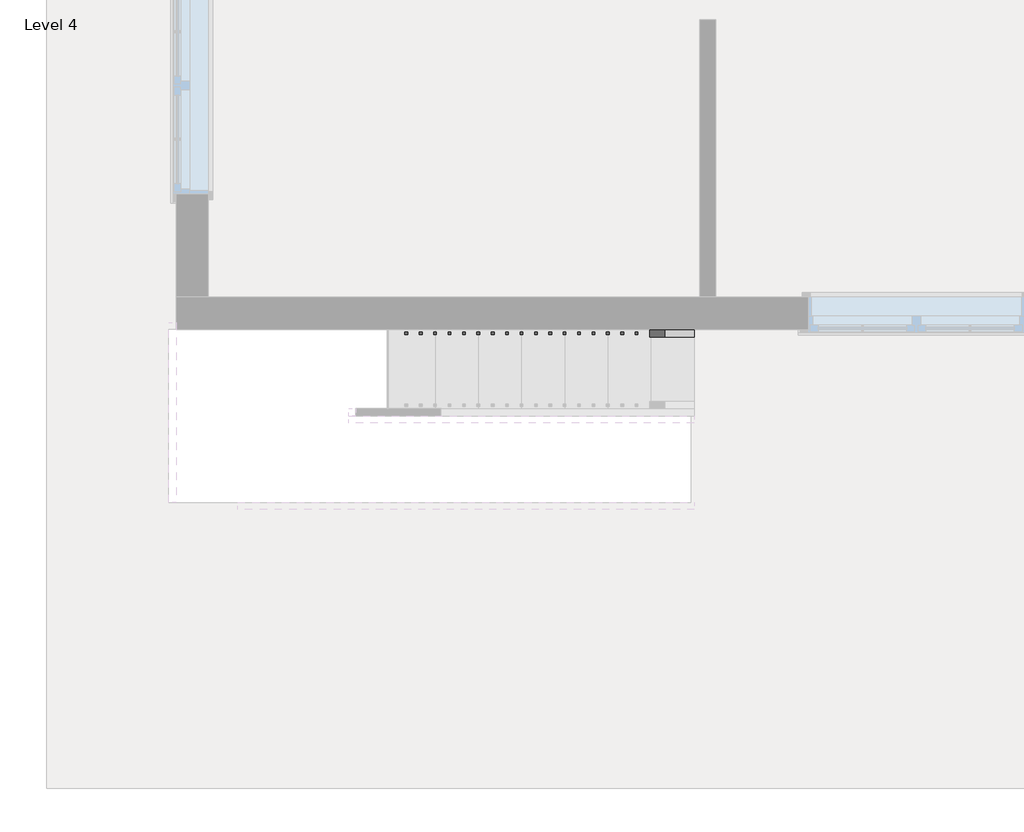
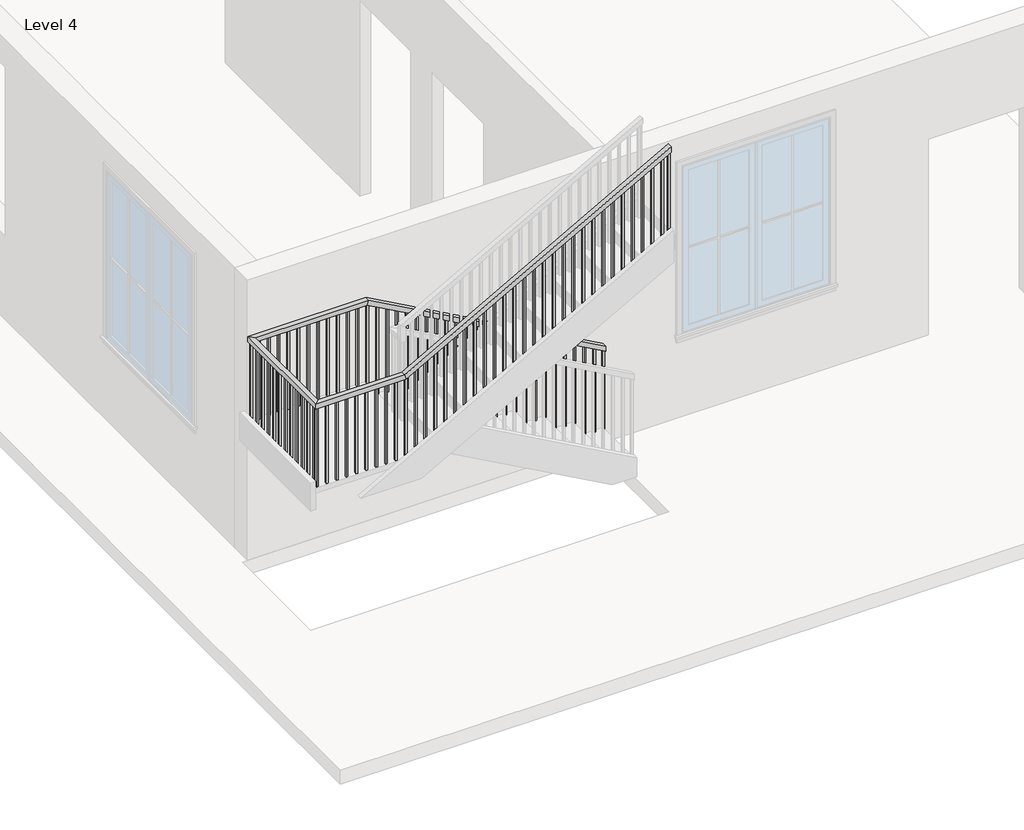
# One storey, part 2 of 3: 1 railing.
"""IFC4 building model written with IfcOpenShell, lengths in millimetres."""

from ifc_helpers import new_model, si_unit, frame, origin, place, context, project, spatial, polyline, outline, extrude, faceted_brep, element, save

model = new_model("IFC4")

# Units and contexts
model_context = context("Model", 3, world=origin())
ifc_project = project(units=[si_unit("LENGTHUNIT", "METRE", prefix="MILLI")], contexts=[model_context])

# Site, building, storey
site = spatial("IfcSite", under=ifc_project)
building = spatial("IfcBuilding", under=site)
storey = spatial("IfcBuildingStorey", under=building, Name="Level 4", Elevation=6400.8)

# Railing
placement = place(None, origin())
element("IfcRailing", 1, ObjectType="Handrail - Rectangular", at=placement, inside=storey, context=model_context, shape_type="SolidModel", body=[
    faceted_brep([(-1805.9198569, -5357.1933037, 7484.5333333), (-1805.9198569, -5357.1933037, 7426.420221), (-1805.9198569, -5306.3933037, 7426.420221), (-1805.9198569, -5306.3933037, 7484.5333333), (-4244.3198569, -5357.1933037, 8839.2), (-4257.4834592, -5357.1933037, 8788.4), (-4257.4834592, -5306.3933037, 8788.4), (-4244.3198569, -5306.3933037, 8839.2), (-5412.7198569, -5357.1933037, 8839.2), (-5412.7198569, -5357.1933037, 8788.4), (-5463.5198569, -5306.3933037, 8788.4), (-5463.5198569, -5306.3933037, 8839.2), (-5412.7198569, -6474.7933037, 8839.2), (-5412.7198569, -6474.7933037, 8788.4), (-5463.5198569, -6525.5933037, 8788.4), (-5463.5198569, -6525.5933037, 8839.2), (-4549.1198569, -6474.7933037, 8839.2), (-4535.9562547, -6474.7933037, 8788.4), (-4535.9562547, -6525.5933037, 8788.4), (-4549.1198569, -6525.5933037, 8839.2), (-1805.9198569, -6474.7933037, 10363.2), (-1805.9198569, -6525.5933037, 10363.2), (-1805.9198569, -6525.5933037, 10305.0868876), (-1805.9198569, -6474.7933037, 10305.0868876)], [[[0, 1, 2, 3]], [[1, 0, 4, 5]], [[2, 1, 5, 6]], [[3, 2, 6, 7]], [[0, 3, 7, 4]], [[5, 4, 8, 9]], [[6, 5, 9, 10]], [[7, 6, 10, 11]], [[4, 7, 11, 8]], [[9, 8, 12, 13]], [[10, 9, 13, 14]], [[11, 10, 14, 15]], [[8, 11, 15, 12]], [[13, 12, 16, 17]], [[14, 13, 17, 18]], [[15, 14, 18, 19]], [[12, 15, 19, 16]], [[20, 21, 22, 23]], [[17, 16, 20, 23]], [[18, 17, 23, 22]], [[19, 18, 22, 21]], [[16, 19, 21, 20]]]),
    extrude(outline(polyline([(10268.045221, -1872.5948569), (10257.4618876, -1891.6448569), (9279.4666667, -1891.6448569), (9279.4666667, -1872.5948569), (10268.045221, -1872.5948569)])), frame((0.0, -6509.7183037, 0.0), z_axis=(0.0, 1.0, 0.0), x_axis=(0.0, 0.0, 1.0)), (0.0, 0.0, 1.0), 19.05),
    extrude(outline(polyline([(10211.6007765, -1974.1948569), (10201.0174432, -1993.2448569), (9279.4666667, -1993.2448569), (9279.4666667, -1974.1948569), (10211.6007765, -1974.1948569)])), frame((0.0, -6509.7183037, 0.0), z_axis=(0.0, 1.0, 0.0), x_axis=(0.0, 0.0, 1.0)), (0.0, 0.0, 1.0), 19.05),
    extrude(outline(polyline([(10155.1563321, -2075.7948569), (10144.5729988, -2094.8448569), (9279.4666667, -2094.8448569), (9279.4666667, -2075.7948569), (10155.1563321, -2075.7948569)])), frame((0.0, -6509.7183037, 0.0), z_axis=(0.0, 1.0, 0.0), x_axis=(0.0, 0.0, 1.0)), (0.0, 0.0, 1.0), 19.05),
    extrude(outline(polyline([(10098.7118876, -2177.3948569), (10088.1285543, -2196.4448569), (9110.1333333, -2196.4448569), (9110.1333333, -2177.3948569), (10098.7118876, -2177.3948569)])), frame((0.0, -6509.7183037, 0.0), z_axis=(0.0, 1.0, 0.0), x_axis=(0.0, 0.0, 1.0)), (0.0, 0.0, 1.0), 19.05),
    extrude(outline(polyline([(10042.2674432, -2278.9948569), (10031.6841099, -2298.0448569), (9110.1333333, -2298.0448569), (9110.1333333, -2278.9948569), (10042.2674432, -2278.9948569)])), frame((0.0, -6509.7183037, 0.0), z_axis=(0.0, 1.0, 0.0), x_axis=(0.0, 0.0, 1.0)), (0.0, 0.0, 1.0), 19.05),
    extrude(outline(polyline([(9985.8229988, -2380.5948569), (9975.2396654, -2399.6448569), (9110.1333333, -2399.6448569), (9110.1333333, -2380.5948569), (9985.8229988, -2380.5948569)])), frame((0.0, -6509.7183037, 0.0), z_axis=(0.0, 1.0, 0.0), x_axis=(0.0, 0.0, 1.0)), (0.0, 0.0, 1.0), 19.05),
    extrude(outline(polyline([(9929.3785543, -2482.1948569), (9918.795221, -2501.2448569), (8940.8, -2501.2448569), (8940.8, -2482.1948569), (9929.3785543, -2482.1948569)])), frame((0.0, -6509.7183037, 0.0), z_axis=(0.0, 1.0, 0.0), x_axis=(0.0, 0.0, 1.0)), (0.0, 0.0, 1.0), 19.05),
    extrude(outline(polyline([(9872.9341099, -2583.7948569), (9862.3507765, -2602.8448569), (8940.8, -2602.8448569), (8940.8, -2583.7948569), (9872.9341099, -2583.7948569)])), frame((0.0, -6509.7183037, 0.0), z_axis=(0.0, 1.0, 0.0), x_axis=(0.0, 0.0, 1.0)), (0.0, 0.0, 1.0), 19.05),
    extrude(outline(polyline([(9816.4896654, -2685.3948569), (9805.9063321, -2704.4448569), (8940.8, -2704.4448569), (8940.8, -2685.3948569), (9816.4896654, -2685.3948569)])), frame((0.0, -6509.7183037, 0.0), z_axis=(0.0, 1.0, 0.0), x_axis=(0.0, 0.0, 1.0)), (0.0, 0.0, 1.0), 19.05),
    extrude(outline(polyline([(9760.045221, -2786.9948569), (9749.4618876, -2806.0448569), (8771.4666667, -2806.0448569), (8771.4666667, -2786.9948569), (9760.045221, -2786.9948569)])), frame((0.0, -6509.7183037, 0.0), z_axis=(0.0, 1.0, 0.0), x_axis=(0.0, 0.0, 1.0)), (0.0, 0.0, 1.0), 19.05),
    extrude(outline(polyline([(9703.6007765, -2888.5948569), (9693.0174432, -2907.6448569), (8771.4666667, -2907.6448569), (8771.4666667, -2888.5948569), (9703.6007765, -2888.5948569)])), frame((0.0, -6509.7183037, 0.0), z_axis=(0.0, 1.0, 0.0), x_axis=(0.0, 0.0, 1.0)), (0.0, 0.0, 1.0), 19.05),
    extrude(outline(polyline([(9647.1563321, -2990.1948569), (9636.5729988, -3009.2448569), (8771.4666667, -3009.2448569), (8771.4666667, -2990.1948569), (9647.1563321, -2990.1948569)])), frame((0.0, -6509.7183037, 0.0), z_axis=(0.0, 1.0, 0.0), x_axis=(0.0, 0.0, 1.0)), (0.0, 0.0, 1.0), 19.05),
    extrude(outline(polyline([(9590.7118876, -3091.7948569), (9580.1285543, -3110.8448569), (8602.1333333, -3110.8448569), (8602.1333333, -3091.7948569), (9590.7118876, -3091.7948569)])), frame((0.0, -6509.7183037, 0.0), z_axis=(0.0, 1.0, 0.0), x_axis=(0.0, 0.0, 1.0)), (0.0, 0.0, 1.0), 19.05),
    extrude(outline(polyline([(9534.2674432, -3193.3948569), (9523.6841099, -3212.4448569), (8602.1333333, -3212.4448569), (8602.1333333, -3193.3948569), (9534.2674432, -3193.3948569)])), frame((0.0, -6509.7183037, 0.0), z_axis=(0.0, 1.0, 0.0), x_axis=(0.0, 0.0, 1.0)), (0.0, 0.0, 1.0), 19.05),
    extrude(outline(polyline([(9477.8229988, -3294.9948569), (9467.2396654, -3314.0448569), (8602.1333333, -3314.0448569), (8602.1333333, -3294.9948569), (9477.8229988, -3294.9948569)])), frame((0.0, -6509.7183037, 0.0), z_axis=(0.0, 1.0, 0.0), x_axis=(0.0, 0.0, 1.0)), (0.0, 0.0, 1.0), 19.05),
    extrude(outline(polyline([(9421.3785543, -3396.5948569), (9410.795221, -3415.6448569), (8432.8, -3415.6448569), (8432.8, -3396.5948569), (9421.3785543, -3396.5948569)])), frame((0.0, -6509.7183037, 0.0), z_axis=(0.0, 1.0, 0.0), x_axis=(0.0, 0.0, 1.0)), (0.0, 0.0, 1.0), 19.05),
    extrude(outline(polyline([(9364.9341099, -3498.1948569), (9354.3507765, -3517.2448569), (8432.8, -3517.2448569), (8432.8, -3498.1948569), (9364.9341099, -3498.1948569)])), frame((0.0, -6509.7183037, 0.0), z_axis=(0.0, 1.0, 0.0), x_axis=(0.0, 0.0, 1.0)), (0.0, 0.0, 1.0), 19.05),
    extrude(outline(polyline([(9308.4896654, -3599.7948569), (9297.9063321, -3618.8448569), (8432.8, -3618.8448569), (8432.8, -3599.7948569), (9308.4896654, -3599.7948569)])), frame((0.0, -6509.7183037, 0.0), z_axis=(0.0, 1.0, 0.0), x_axis=(0.0, 0.0, 1.0)), (0.0, 0.0, 1.0), 19.05),
    extrude(outline(polyline([(9252.045221, -3701.3948569), (9241.4618876, -3720.4448569), (8263.4666667, -3720.4448569), (8263.4666667, -3701.3948569), (9252.045221, -3701.3948569)])), frame((0.0, -6509.7183037, 0.0), z_axis=(0.0, 1.0, 0.0), x_axis=(0.0, 0.0, 1.0)), (0.0, 0.0, 1.0), 19.05),
    extrude(outline(polyline([(9195.6007765, -3802.9948569), (9185.0174432, -3822.0448569), (8263.4666667, -3822.0448569), (8263.4666667, -3802.9948569), (9195.6007765, -3802.9948569)])), frame((0.0, -6509.7183037, 0.0), z_axis=(0.0, 1.0, 0.0), x_axis=(0.0, 0.0, 1.0)), (0.0, 0.0, 1.0), 19.05),
    extrude(outline(polyline([(9139.1563321, -3904.5948569), (9128.5729988, -3923.6448569), (8263.4666667, -3923.6448569), (8263.4666667, -3904.5948569), (9139.1563321, -3904.5948569)])), frame((0.0, -6509.7183037, 0.0), z_axis=(0.0, 1.0, 0.0), x_axis=(0.0, 0.0, 1.0)), (0.0, 0.0, 1.0), 19.05),
    extrude(outline(polyline([(9082.7118876, -4006.1948569), (9072.1285543, -4025.2448569), (8094.1333333, -4025.2448569), (8094.1333333, -4006.1948569), (9082.7118876, -4006.1948569)])), frame((0.0, -6509.7183037, 0.0), z_axis=(0.0, 1.0, 0.0), x_axis=(0.0, 0.0, 1.0)), (0.0, 0.0, 1.0), 19.05),
    extrude(outline(polyline([(9026.2674432, -4107.7948569), (9015.6841099, -4126.8448569), (8094.1333333, -4126.8448569), (8094.1333333, -4107.7948569), (9026.2674432, -4107.7948569)])), frame((0.0, -6509.7183037, 0.0), z_axis=(0.0, 1.0, 0.0), x_axis=(0.0, 0.0, 1.0)), (0.0, 0.0, 1.0), 19.05),
    extrude(outline(polyline([(8969.8229988, -4209.3948569), (8959.2396654, -4228.4448569), (8094.1333333, -4228.4448569), (8094.1333333, -4209.3948569), (8969.8229988, -4209.3948569)])), frame((0.0, -6509.7183037, 0.0), z_axis=(0.0, 1.0, 0.0), x_axis=(0.0, 0.0, 1.0)), (0.0, 0.0, 1.0), 19.05),
    extrude(outline(polyline([(8913.3785543, -4310.9948569), (8902.795221, -4330.0448569), (7924.8, -4330.0448569), (7924.8, -4310.9948569), (8913.3785543, -4310.9948569)])), frame((0.0, -6509.7183037, 0.0), z_axis=(0.0, 1.0, 0.0), x_axis=(0.0, 0.0, 1.0)), (0.0, 0.0, 1.0), 19.05),
    extrude(outline(polyline([(8856.9341099, -4412.5948569), (8846.3507765, -4431.6448569), (7924.8, -4431.6448569), (7924.8, -4412.5948569), (8856.9341099, -4412.5948569)])), frame((0.0, -6509.7183037, 0.0), z_axis=(0.0, 1.0, 0.0), x_axis=(0.0, 0.0, 1.0)), (0.0, 0.0, 1.0), 19.05),
    extrude(outline(polyline([(8800.4896654, -4514.1948569), (8789.9063321, -4533.2448569), (7924.8, -4533.2448569), (7924.8, -4514.1948569), (8800.4896654, -4514.1948569)])), frame((0.0, -6509.7183037, 0.0), z_axis=(0.0, 1.0, 0.0), x_axis=(0.0, 0.0, 1.0)), (0.0, 0.0, 1.0), 19.05),
    extrude(outline(polyline([(-4634.8448569, -6509.7183037), (-4634.8448569, -6490.6683037), (-4615.7948569, -6490.6683037), (-4615.7948569, -6509.7183037), (-4634.8448569, -6509.7183037)])), frame((0.0, 0.0, 7924.8), z_axis=(0.0, 0.0, 1.0), x_axis=(1.0, 0.0, 0.0)), (0.0, 0.0, 1.0), 863.6),
    extrude(outline(polyline([(-4736.4448569, -6509.7183037), (-4736.4448569, -6490.6683037), (-4717.3948569, -6490.6683037), (-4717.3948569, -6509.7183037), (-4736.4448569, -6509.7183037)])), frame((0.0, 0.0, 7924.8), z_axis=(0.0, 0.0, 1.0), x_axis=(1.0, 0.0, 0.0)), (0.0, 0.0, 1.0), 863.6),
    extrude(outline(polyline([(-4838.0448569, -6509.7183037), (-4838.0448569, -6490.6683037), (-4818.9948569, -6490.6683037), (-4818.9948569, -6509.7183037), (-4838.0448569, -6509.7183037)])), frame((0.0, 0.0, 7924.8), z_axis=(0.0, 0.0, 1.0), x_axis=(1.0, 0.0, 0.0)), (0.0, 0.0, 1.0), 863.6),
    extrude(outline(polyline([(-4939.6448569, -6509.7183037), (-4939.6448569, -6490.6683037), (-4920.5948569, -6490.6683037), (-4920.5948569, -6509.7183037), (-4939.6448569, -6509.7183037)])), frame((0.0, 0.0, 7924.8), z_axis=(0.0, 0.0, 1.0), x_axis=(1.0, 0.0, 0.0)), (0.0, 0.0, 1.0), 863.6),
    extrude(outline(polyline([(-5041.2448569, -6509.7183037), (-5041.2448569, -6490.6683037), (-5022.1948569, -6490.6683037), (-5022.1948569, -6509.7183037), (-5041.2448569, -6509.7183037)])), frame((0.0, 0.0, 7924.8), z_axis=(0.0, 0.0, 1.0), x_axis=(1.0, 0.0, 0.0)), (0.0, 0.0, 1.0), 863.6),
    extrude(outline(polyline([(-5142.8448569, -6509.7183037), (-5142.8448569, -6490.6683037), (-5123.7948569, -6490.6683037), (-5123.7948569, -6509.7183037), (-5142.8448569, -6509.7183037)])), frame((0.0, 0.0, 7924.8), z_axis=(0.0, 0.0, 1.0), x_axis=(1.0, 0.0, 0.0)), (0.0, 0.0, 1.0), 863.6),
    extrude(outline(polyline([(-5244.4448569, -6509.7183037), (-5244.4448569, -6490.6683037), (-5225.3948569, -6490.6683037), (-5225.3948569, -6509.7183037), (-5244.4448569, -6509.7183037)])), frame((0.0, 0.0, 7924.8), z_axis=(0.0, 0.0, 1.0), x_axis=(1.0, 0.0, 0.0)), (0.0, 0.0, 1.0), 863.6),
    extrude(outline(polyline([(-5346.0448569, -6509.7183037), (-5346.0448569, -6490.6683037), (-5326.9948569, -6490.6683037), (-5326.9948569, -6509.7183037), (-5346.0448569, -6509.7183037)])), frame((0.0, 0.0, 7924.8), z_axis=(0.0, 0.0, 1.0), x_axis=(1.0, 0.0, 0.0)), (0.0, 0.0, 1.0), 863.6),
    extrude(outline(polyline([(-5447.6448569, -6439.8683037), (-5428.5948569, -6439.8683037), (-5428.5948569, -6458.9183037), (-5447.6448569, -6458.9183037), (-5447.6448569, -6439.8683037)])), frame((0.0, 0.0, 7924.8), z_axis=(0.0, 0.0, 1.0), x_axis=(1.0, 0.0, 0.0)), (0.0, 0.0, 1.0), 863.6),
    extrude(outline(polyline([(-5447.6448569, -6338.2683037), (-5428.5948569, -6338.2683037), (-5428.5948569, -6357.3183037), (-5447.6448569, -6357.3183037), (-5447.6448569, -6338.2683037)])), frame((0.0, 0.0, 7924.8), z_axis=(0.0, 0.0, 1.0), x_axis=(1.0, 0.0, 0.0)), (0.0, 0.0, 1.0), 863.6),
    extrude(outline(polyline([(-5447.6448569, -6236.6683037), (-5428.5948569, -6236.6683037), (-5428.5948569, -6255.7183037), (-5447.6448569, -6255.7183037), (-5447.6448569, -6236.6683037)])), frame((0.0, 0.0, 7924.8), z_axis=(0.0, 0.0, 1.0), x_axis=(1.0, 0.0, 0.0)), (0.0, 0.0, 1.0), 863.6),
    extrude(outline(polyline([(-5447.6448569, -6135.0683037), (-5428.5948569, -6135.0683037), (-5428.5948569, -6154.1183037), (-5447.6448569, -6154.1183037), (-5447.6448569, -6135.0683037)])), frame((0.0, 0.0, 7924.8), z_axis=(0.0, 0.0, 1.0), x_axis=(1.0, 0.0, 0.0)), (0.0, 0.0, 1.0), 863.6),
    extrude(outline(polyline([(-5447.6448569, -6033.4683037), (-5428.5948569, -6033.4683037), (-5428.5948569, -6052.5183037), (-5447.6448569, -6052.5183037), (-5447.6448569, -6033.4683037)])), frame((0.0, 0.0, 7924.8), z_axis=(0.0, 0.0, 1.0), x_axis=(1.0, 0.0, 0.0)), (0.0, 0.0, 1.0), 863.6),
    extrude(outline(polyline([(-5447.6448569, -5931.8683037), (-5428.5948569, -5931.8683037), (-5428.5948569, -5950.9183037), (-5447.6448569, -5950.9183037), (-5447.6448569, -5931.8683037)])), frame((0.0, 0.0, 7924.8), z_axis=(0.0, 0.0, 1.0), x_axis=(1.0, 0.0, 0.0)), (0.0, 0.0, 1.0), 863.6),
    extrude(outline(polyline([(-5447.6448569, -5830.2683037), (-5428.5948569, -5830.2683037), (-5428.5948569, -5849.3183037), (-5447.6448569, -5849.3183037), (-5447.6448569, -5830.2683037)])), frame((0.0, 0.0, 7924.8), z_axis=(0.0, 0.0, 1.0), x_axis=(1.0, 0.0, 0.0)), (0.0, 0.0, 1.0), 863.6),
    extrude(outline(polyline([(-5447.6448569, -5728.6683037), (-5428.5948569, -5728.6683037), (-5428.5948569, -5747.7183037), (-5447.6448569, -5747.7183037), (-5447.6448569, -5728.6683037)])), frame((0.0, 0.0, 7924.8), z_axis=(0.0, 0.0, 1.0), x_axis=(1.0, 0.0, 0.0)), (0.0, 0.0, 1.0), 863.6),
    extrude(outline(polyline([(-5447.6448569, -5627.0683037), (-5428.5948569, -5627.0683037), (-5428.5948569, -5646.1183037), (-5447.6448569, -5646.1183037), (-5447.6448569, -5627.0683037)])), frame((0.0, 0.0, 7924.8), z_axis=(0.0, 0.0, 1.0), x_axis=(1.0, 0.0, 0.0)), (0.0, 0.0, 1.0), 863.6),
    extrude(outline(polyline([(-5447.6448569, -5525.4683037), (-5428.5948569, -5525.4683037), (-5428.5948569, -5544.5183037), (-5447.6448569, -5544.5183037), (-5447.6448569, -5525.4683037)])), frame((0.0, 0.0, 7924.8), z_axis=(0.0, 0.0, 1.0), x_axis=(1.0, 0.0, 0.0)), (0.0, 0.0, 1.0), 863.6),
    extrude(outline(polyline([(-5447.6448569, -5423.8683037), (-5428.5948569, -5423.8683037), (-5428.5948569, -5442.9183037), (-5447.6448569, -5442.9183037), (-5447.6448569, -5423.8683037)])), frame((0.0, 0.0, 7924.8), z_axis=(0.0, 0.0, 1.0), x_axis=(1.0, 0.0, 0.0)), (0.0, 0.0, 1.0), 863.6),
    extrude(outline(polyline([(-5352.3948569, -5322.2683037), (-5352.3948569, -5341.3183037), (-5371.4448569, -5341.3183037), (-5371.4448569, -5322.2683037), (-5352.3948569, -5322.2683037)])), frame((0.0, 0.0, 7924.8), z_axis=(0.0, 0.0, 1.0), x_axis=(1.0, 0.0, 0.0)), (0.0, 0.0, 1.0), 863.6),
    extrude(outline(polyline([(-5250.7948569, -5322.2683037), (-5250.7948569, -5341.3183037), (-5269.8448569, -5341.3183037), (-5269.8448569, -5322.2683037), (-5250.7948569, -5322.2683037)])), frame((0.0, 0.0, 7924.8), z_axis=(0.0, 0.0, 1.0), x_axis=(1.0, 0.0, 0.0)), (0.0, 0.0, 1.0), 863.6),
    extrude(outline(polyline([(-5149.1948569, -5322.2683037), (-5149.1948569, -5341.3183037), (-5168.2448569, -5341.3183037), (-5168.2448569, -5322.2683037), (-5149.1948569, -5322.2683037)])), frame((0.0, 0.0, 7924.8), z_axis=(0.0, 0.0, 1.0), x_axis=(1.0, 0.0, 0.0)), (0.0, 0.0, 1.0), 863.6),
    extrude(outline(polyline([(-5047.5948569, -5322.2683037), (-5047.5948569, -5341.3183037), (-5066.6448569, -5341.3183037), (-5066.6448569, -5322.2683037), (-5047.5948569, -5322.2683037)])), frame((0.0, 0.0, 7924.8), z_axis=(0.0, 0.0, 1.0), x_axis=(1.0, 0.0, 0.0)), (0.0, 0.0, 1.0), 863.6),
    extrude(outline(polyline([(-4945.9948569, -5322.2683037), (-4945.9948569, -5341.3183037), (-4965.0448569, -5341.3183037), (-4965.0448569, -5322.2683037), (-4945.9948569, -5322.2683037)])), frame((0.0, 0.0, 7924.8), z_axis=(0.0, 0.0, 1.0), x_axis=(1.0, 0.0, 0.0)), (0.0, 0.0, 1.0), 863.6),
    extrude(outline(polyline([(-4844.3948569, -5322.2683037), (-4844.3948569, -5341.3183037), (-4863.4448569, -5341.3183037), (-4863.4448569, -5322.2683037), (-4844.3948569, -5322.2683037)])), frame((0.0, 0.0, 7924.8), z_axis=(0.0, 0.0, 1.0), x_axis=(1.0, 0.0, 0.0)), (0.0, 0.0, 1.0), 863.6),
    extrude(outline(polyline([(-4742.7948569, -5322.2683037), (-4742.7948569, -5341.3183037), (-4761.8448569, -5341.3183037), (-4761.8448569, -5322.2683037), (-4742.7948569, -5322.2683037)])), frame((0.0, 0.0, 7924.8), z_axis=(0.0, 0.0, 1.0), x_axis=(1.0, 0.0, 0.0)), (0.0, 0.0, 1.0), 863.6),
    extrude(outline(polyline([(-4641.1948569, -5322.2683037), (-4641.1948569, -5341.3183037), (-4660.2448569, -5341.3183037), (-4660.2448569, -5322.2683037), (-4641.1948569, -5322.2683037)])), frame((0.0, 0.0, 7924.8), z_axis=(0.0, 0.0, 1.0), x_axis=(1.0, 0.0, 0.0)), (0.0, 0.0, 1.0), 863.6),
    extrude(outline(polyline([(-4539.5948569, -5322.2683037), (-4539.5948569, -5341.3183037), (-4558.6448569, -5341.3183037), (-4558.6448569, -5322.2683037), (-4539.5948569, -5322.2683037)])), frame((0.0, 0.0, 7924.8), z_axis=(0.0, 0.0, 1.0), x_axis=(1.0, 0.0, 0.0)), (0.0, 0.0, 1.0), 863.6),
    extrude(outline(polyline([(-4437.9948569, -5322.2683037), (-4437.9948569, -5341.3183037), (-4457.0448569, -5341.3183037), (-4457.0448569, -5322.2683037), (-4437.9948569, -5322.2683037)])), frame((0.0, 0.0, 7924.8), z_axis=(0.0, 0.0, 1.0), x_axis=(1.0, 0.0, 0.0)), (0.0, 0.0, 1.0), 863.6),
    extrude(outline(polyline([(-4336.3948569, -5322.2683037), (-4336.3948569, -5341.3183037), (-4355.4448569, -5341.3183037), (-4355.4448569, -5322.2683037), (-4336.3948569, -5322.2683037)])), frame((0.0, 0.0, 7924.8), z_axis=(0.0, 0.0, 1.0), x_axis=(1.0, 0.0, 0.0)), (0.0, 0.0, 1.0), 863.6),
    extrude(outline(polyline([(8775.795221, -4234.7948569), (8786.3785543, -4253.8448569), (7924.8, -4253.8448569), (7924.8, -4234.7948569), (8775.795221, -4234.7948569)])), frame((0.0, -5341.3183037, 0.0), z_axis=(0.0, 1.0, 0.0), x_axis=(0.0, 0.0, 1.0)), (0.0, 0.0, 1.0), 19.05),
    extrude(outline(polyline([(8719.3507765, -4133.1948569), (8729.9341099, -4152.2448569), (7755.4666667, -4152.2448569), (7755.4666667, -4133.1948569), (8719.3507765, -4133.1948569)])), frame((0.0, -5341.3183037, 0.0), z_axis=(0.0, 1.0, 0.0), x_axis=(0.0, 0.0, 1.0)), (0.0, 0.0, 1.0), 19.05),
    extrude(outline(polyline([(8662.9063321, -4031.5948569), (8673.4896654, -4050.6448569), (7755.4666667, -4050.6448569), (7755.4666667, -4031.5948569), (8662.9063321, -4031.5948569)])), frame((0.0, -5341.3183037, 0.0), z_axis=(0.0, 1.0, 0.0), x_axis=(0.0, 0.0, 1.0)), (0.0, 0.0, 1.0), 19.05),
    extrude(outline(polyline([(8606.4618876, -3929.9948569), (8617.045221, -3949.0448569), (7755.4666667, -3949.0448569), (7755.4666667, -3929.9948569), (8606.4618876, -3929.9948569)])), frame((0.0, -5341.3183037, 0.0), z_axis=(0.0, 1.0, 0.0), x_axis=(0.0, 0.0, 1.0)), (0.0, 0.0, 1.0), 19.05),
    extrude(outline(polyline([(8550.0174432, -3828.3948569), (8560.6007765, -3847.4448569), (7586.1333333, -3847.4448569), (7586.1333333, -3828.3948569), (8550.0174432, -3828.3948569)])), frame((0.0, -5341.3183037, 0.0), z_axis=(0.0, 1.0, 0.0), x_axis=(0.0, 0.0, 1.0)), (0.0, 0.0, 1.0), 19.05),
    extrude(outline(polyline([(8493.5729988, -3726.7948569), (8504.1563321, -3745.8448569), (7586.1333333, -3745.8448569), (7586.1333333, -3726.7948569), (8493.5729988, -3726.7948569)])), frame((0.0, -5341.3183037, 0.0), z_axis=(0.0, 1.0, 0.0), x_axis=(0.0, 0.0, 1.0)), (0.0, 0.0, 1.0), 19.05),
    extrude(outline(polyline([(8437.1285543, -3625.1948569), (8447.7118876, -3644.2448569), (7586.1333333, -3644.2448569), (7586.1333333, -3625.1948569), (8437.1285543, -3625.1948569)])), frame((0.0, -5341.3183037, 0.0), z_axis=(0.0, 1.0, 0.0), x_axis=(0.0, 0.0, 1.0)), (0.0, 0.0, 1.0), 19.05),
    extrude(outline(polyline([(8380.6841099, -3523.5948569), (8391.2674432, -3542.6448569), (7416.8, -3542.6448569), (7416.8, -3523.5948569), (8380.6841099, -3523.5948569)])), frame((0.0, -5341.3183037, 0.0), z_axis=(0.0, 1.0, 0.0), x_axis=(0.0, 0.0, 1.0)), (0.0, 0.0, 1.0), 19.05),
    extrude(outline(polyline([(8324.2396654, -3421.9948569), (8334.8229988, -3441.0448569), (7416.8, -3441.0448569), (7416.8, -3421.9948569), (8324.2396654, -3421.9948569)])), frame((0.0, -5341.3183037, 0.0), z_axis=(0.0, 1.0, 0.0), x_axis=(0.0, 0.0, 1.0)), (0.0, 0.0, 1.0), 19.05),
    extrude(outline(polyline([(8267.795221, -3320.3948569), (8278.3785543, -3339.4448569), (7416.8, -3339.4448569), (7416.8, -3320.3948569), (8267.795221, -3320.3948569)])), frame((0.0, -5341.3183037, 0.0), z_axis=(0.0, 1.0, 0.0), x_axis=(0.0, 0.0, 1.0)), (0.0, 0.0, 1.0), 19.05),
    extrude(outline(polyline([(8211.3507765, -3218.7948569), (8221.9341099, -3237.8448569), (7247.4666667, -3237.8448569), (7247.4666667, -3218.7948569), (8211.3507765, -3218.7948569)])), frame((0.0, -5341.3183037, 0.0), z_axis=(0.0, 1.0, 0.0), x_axis=(0.0, 0.0, 1.0)), (0.0, 0.0, 1.0), 19.05),
    extrude(outline(polyline([(8154.9063321, -3117.1948569), (8165.4896654, -3136.2448569), (7247.4666667, -3136.2448569), (7247.4666667, -3117.1948569), (8154.9063321, -3117.1948569)])), frame((0.0, -5341.3183037, 0.0), z_axis=(0.0, 1.0, 0.0), x_axis=(0.0, 0.0, 1.0)), (0.0, 0.0, 1.0), 19.05),
    extrude(outline(polyline([(8098.4618876, -3015.5948569), (8109.045221, -3034.6448569), (7247.4666667, -3034.6448569), (7247.4666667, -3015.5948569), (8098.4618876, -3015.5948569)])), frame((0.0, -5341.3183037, 0.0), z_axis=(0.0, 1.0, 0.0), x_axis=(0.0, 0.0, 1.0)), (0.0, 0.0, 1.0), 19.05),
    extrude(outline(polyline([(8042.0174432, -2913.9948569), (8052.6007765, -2933.0448569), (7078.1333333, -2933.0448569), (7078.1333333, -2913.9948569), (8042.0174432, -2913.9948569)])), frame((0.0, -5341.3183037, 0.0), z_axis=(0.0, 1.0, 0.0), x_axis=(0.0, 0.0, 1.0)), (0.0, 0.0, 1.0), 19.05),
    extrude(outline(polyline([(7985.5729988, -2812.3948569), (7996.1563321, -2831.4448569), (7078.1333333, -2831.4448569), (7078.1333333, -2812.3948569), (7985.5729988, -2812.3948569)])), frame((0.0, -5341.3183037, 0.0), z_axis=(0.0, 1.0, 0.0), x_axis=(0.0, 0.0, 1.0)), (0.0, 0.0, 1.0), 19.05),
    extrude(outline(polyline([(7929.1285543, -2710.7948569), (7939.7118876, -2729.8448569), (7078.1333333, -2729.8448569), (7078.1333333, -2710.7948569), (7929.1285543, -2710.7948569)])), frame((0.0, -5341.3183037, 0.0), z_axis=(0.0, 1.0, 0.0), x_axis=(0.0, 0.0, 1.0)), (0.0, 0.0, 1.0), 19.05),
    extrude(outline(polyline([(7872.6841099, -2609.1948569), (7883.2674432, -2628.2448569), (6908.8, -2628.2448569), (6908.8, -2609.1948569), (7872.6841099, -2609.1948569)])), frame((0.0, -5341.3183037, 0.0), z_axis=(0.0, 1.0, 0.0), x_axis=(0.0, 0.0, 1.0)), (0.0, 0.0, 1.0), 19.05),
    extrude(outline(polyline([(7816.2396654, -2507.5948569), (7826.8229988, -2526.6448569), (6908.8, -2526.6448569), (6908.8, -2507.5948569), (7816.2396654, -2507.5948569)])), frame((0.0, -5341.3183037, 0.0), z_axis=(0.0, 1.0, 0.0), x_axis=(0.0, 0.0, 1.0)), (0.0, 0.0, 1.0), 19.05),
    extrude(outline(polyline([(7759.795221, -2405.9948569), (7770.3785543, -2425.0448569), (6908.8, -2425.0448569), (6908.8, -2405.9948569), (7759.795221, -2405.9948569)])), frame((0.0, -5341.3183037, 0.0), z_axis=(0.0, 1.0, 0.0), x_axis=(0.0, 0.0, 1.0)), (0.0, 0.0, 1.0), 19.05),
    extrude(outline(polyline([(7703.3507765, -2304.3948569), (7713.9341099, -2323.4448569), (6739.4666667, -2323.4448569), (6739.4666667, -2304.3948569), (7703.3507765, -2304.3948569)])), frame((0.0, -5341.3183037, 0.0), z_axis=(0.0, 1.0, 0.0), x_axis=(0.0, 0.0, 1.0)), (0.0, 0.0, 1.0), 19.05),
    extrude(outline(polyline([(7646.9063321, -2202.7948569), (7657.4896654, -2221.8448569), (6739.4666667, -2221.8448569), (6739.4666667, -2202.7948569), (7646.9063321, -2202.7948569)])), frame((0.0, -5341.3183037, 0.0), z_axis=(0.0, 1.0, 0.0), x_axis=(0.0, 0.0, 1.0)), (0.0, 0.0, 1.0), 19.05),
    extrude(outline(polyline([(7590.4618876, -2101.1948569), (7601.045221, -2120.2448569), (6739.4666667, -2120.2448569), (6739.4666667, -2101.1948569), (7590.4618876, -2101.1948569)])), frame((0.0, -5341.3183037, 0.0), z_axis=(0.0, 1.0, 0.0), x_axis=(0.0, 0.0, 1.0)), (0.0, 0.0, 1.0), 19.05),
    extrude(outline(polyline([(7534.0174432, -1999.5948569), (7544.6007765, -2018.6448569), (6570.1333333, -2018.6448569), (6570.1333333, -1999.5948569), (7534.0174432, -1999.5948569)])), frame((0.0, -5341.3183037, 0.0), z_axis=(0.0, 1.0, 0.0), x_axis=(0.0, 0.0, 1.0)), (0.0, 0.0, 1.0), 19.05),
    extrude(outline(polyline([(7477.5729988, -1897.9948569), (7488.1563321, -1917.0448569), (6570.1333333, -1917.0448569), (6570.1333333, -1897.9948569), (7477.5729988, -1897.9948569)])), frame((0.0, -5341.3183037, 0.0), z_axis=(0.0, 1.0, 0.0), x_axis=(0.0, 0.0, 1.0)), (0.0, 0.0, 1.0), 19.05),
    extrude(outline(polyline([(-5447.6448569, -6490.6683037), (-5428.5948569, -6490.6683037), (-5428.5948569, -6509.7183037), (-5447.6448569, -6509.7183037), (-5447.6448569, -6490.6683037)])), frame((0.0, 0.0, 7924.8), z_axis=(0.0, 0.0, 1.0), x_axis=(1.0, 0.0, 0.0)), (0.0, 0.0, 1.0), 863.6),
    extrude(outline(polyline([(-5428.5948569, -5322.2683037), (-5428.5948569, -5341.3183037), (-5447.6448569, -5341.3183037), (-5447.6448569, -5322.2683037), (-5428.5948569, -5322.2683037)])), frame((0.0, 0.0, 7924.8), z_axis=(0.0, 0.0, 1.0), x_axis=(1.0, 0.0, 0.0)), (0.0, 0.0, 1.0), 863.6),
    extrude(outline(polyline([(10305.0868876, -1805.9198569), (10294.5035543, -1824.9698569), (9279.4666667, -1824.9698569), (9279.4666667, -1805.9198569), (10305.0868876, -1805.9198569)])), frame((0.0, -6509.7183037, 0.0), z_axis=(0.0, 1.0, 0.0), x_axis=(0.0, 0.0, 1.0)), (0.0, 0.0, 1.0), 19.05),
    extrude(outline(polyline([(7426.420221, -1805.9198569), (7437.0035543, -1824.9698569), (6570.1333333, -1824.9698569), (6570.1333333, -1805.9198569), (7426.420221, -1805.9198569)])), frame((0.0, -5341.3183037, 0.0), z_axis=(0.0, 1.0, 0.0), x_axis=(0.0, 0.0, 1.0)), (0.0, 0.0, 1.0), 19.05),
])

save(model, "model.ifc")

# Revit data of these elements
# Type "Handrail - Rectangular"
#   Assembly Code = "C2010400"
#   built-in parameter 1008612 = 0.0416667 (stored number, unit not read)
#   built-in parameter 1008611 = 0.0416667 (stored number, unit not read)
#   built-in parameter 1008609 = 0.333333 (stored number, unit not read)
#   built-in parameter 1008604 = 0.166667 (stored number, unit not read)
#   built-in parameter 1008603 = 0.166667 (stored number, unit not read)
#   Railing Height = 3' - 0"
#   built-in parameter 1008630 = 2
#   built-in parameter 1008610 = 2
#   built-in parameter 1008618 = Baluster - Square : 3/4"
# Element 1 (IfcRailing, "Handrail - Rectangular")
#   Phase Created = New Construction
